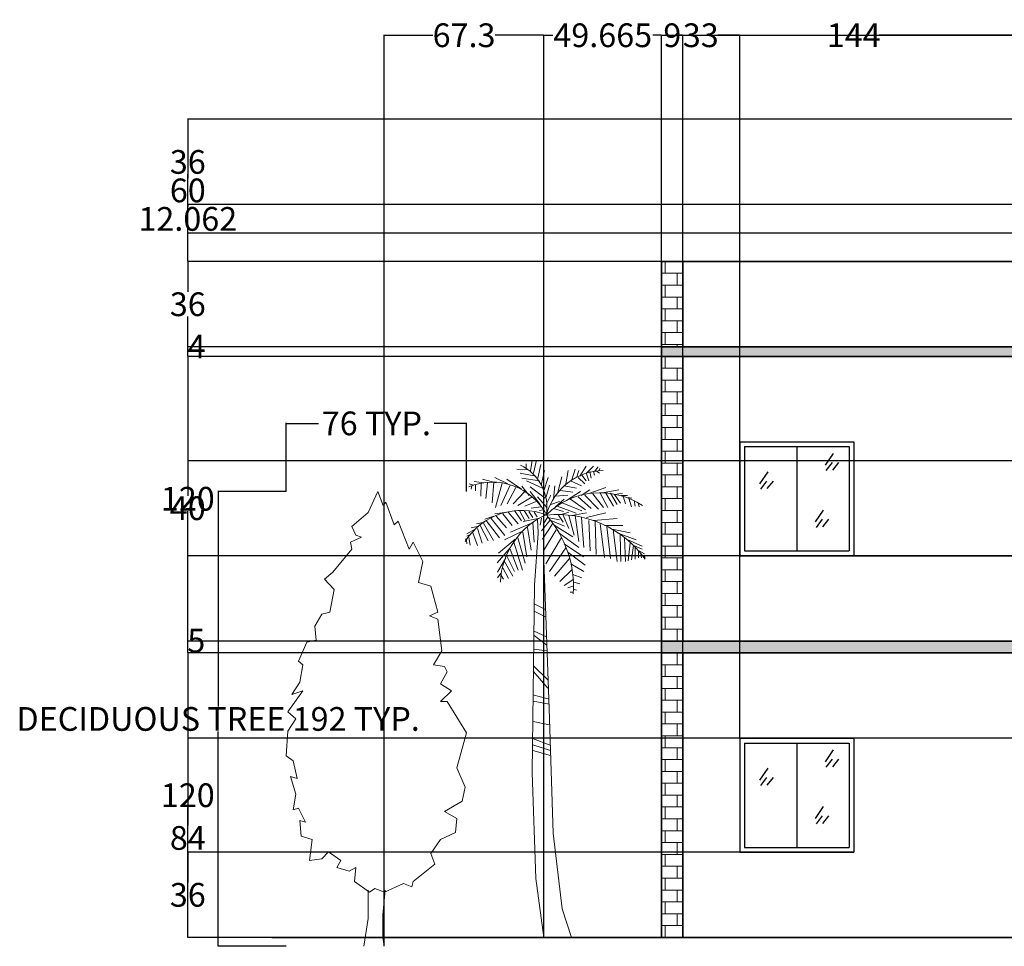
# Model space of a CAD drawing. Units: inches. Extents: x 403 to 1256, y 451 to 842.
# Tile 1 of 4: x 403 to 818, y 451 to 842. Entities that reach past the tile are written whole.
import ezdxf

# ---------------------------------------------------------------- set-up
doc = ezdxf.new("R2010")
doc.units = ezdxf.units.IN
doc.header["$MEASUREMENT"] = 0
for name, color, linetype, lineweight in [('A-ANNO-DIMS', 2, 'Continuous', 18), ('A-GLAZ', 4, 'Continuous', 25), ('A-WALL', 7, 'Continuous', 35), ('A-WALL-PATT', 8, 'Continuous', 13), ('PLANTS', 3, 'Continuous', 18)]:
    doc.layers.add(name, color=color, linetype=linetype, lineweight=lineweight)
doc.styles.get("Standard").update_dxf_attribs({"font": 'arial.ttf'})
doc.dimstyles.get("Standard").update_dxf_attribs({"dimtxt": 10, "dimasz": 0.18, "dimexe": 0.18, "dimexo": 0.0625, "dimgap": 0.09, "dimtad": 0, "dimtih": 1, "dimtoh": 1, "dimdec": 0, "dimzin": 0, "dimdsep": 46, "dimlunit": 3, "dimtxsty": 'Standard', "dimcen": 0.09, "dimadec": 0, "dimazin": 0, "dimtfac": 1, "dimtdec": 0, "dimtofl": 0, "dimtmove": 0, "dimatfit": 3, "dimfxl": 1, "dimtolj": 1, "dimtzin": 0, "dimarcsym": 0})
pattern_1 = [(50, (0, 0), (6.455342, -0.56477), [0.675, -7.425]), (355, (0, 0), (-1.248762, 6.76973), [0.54, -5.94]), (100.45144, (0.538, -0.047), (5.20658, 6.20496), [0.573662, -6.31028]), (46.1842, (0, 1.8), (9.60517, -1.489674), [1.0125, -11.1375]), (96.6356, (0.8, 1.676), (8.41196, 8.76707), [0.86049, -9.465424]), (351.1842, (0, 1.8), (8.41196, 8.76707), [0.81, -8.91]), (21, (0.9, 1.35), (5.372163, -3.62357), [0.675, -7.425]), (326, (0.9, 1.35), (2.189838, 6.52635), [0.54, -5.94]), (71.45144, (1.3477, 1.048), (7.562, 2.90278), [0.573662, -6.31028]), (37.5, (0, 0), (0.1094387, 2.9960447), [0, -5.868, 0, -6.03, 0, -5.9625]), (7.5, (0, 0), (2.367626, 3.549705), [0, -3.438, 0, -5.733, 0, -2.2725]), (327.5, (-2.007, 0), (4.804402, -0.202994), [0, -2.25, 0, -7.02, 0, -9.315]), (317.5, (-2.907, 0), (5.248676, 0.900945), [0, -2.925, 0, -4.662, 0, -6.615])]

# ---------------------------------------------------------------- blocks, each defined once
blk = doc.blocks.new('Tree - palm elevation')
for p, q in [((-7.5, 199.68), (-7.5, 197.946)), ((-5.567, 196.707), (-4.987, 201.167)), ((-4.407, 195.716), (-3.247, 200.672)), ((-2.474, 193.733), (-1.315, 199.433)), ((-6.727, 197.202), (-11.366, 197.45)), ((-3.441, 194.477), (-10.013, 195.716)), ((-1.121, 190.759), (0.232, 196.955)), ((9.317, 191.255), (10.283, 196.955)), ((11.829, 192.99), (13.182, 197.45)), ((13.956, 194.229), (14.729, 196.955)), ((15.116, 194.477), (17.822, 198.689)), ((18.015, 195.716), (20.914, 198.689)), ((18.015, 195.468), (18.981, 192.494)), ((19.368, 196.459), (19.948, 193.733)), ((20.914, 196.459), (21.301, 194.972)), ((21.301, 196.459), (22.847, 198.441)), ((22.074, 196.707), (23.427, 195.716)), ((23.234, 196.707), (23.62, 197.698)), ((-29.729, 190.759), (-31.469, 191.255)), ((-25.283, 191.751), (-29.342, 192.246)), ((-26.443, 191.503), (-26.636, 186.051)), ((-20.064, 191.751), (-25.863, 193.238)), ((-23.737, 191.751), (-24.51, 185.06)), ((-21.031, 191.998), (-21.804, 183.325)), ((-15.232, 191.255), (-20.644, 193.981)), ((-17.551, 191.503), (-20.451, 181.343)), ((-9.433, 189.025), (-15.618, 193.238)), ((-1.894, 192.494), (-9.24, 193.733)), ((-0.541, 189.52), (-7.307, 192.494)), ((0.038, 188.281), (1.778, 193.981)), ((5.837, 187.786), (7.577, 194.229)), ((11.25, 192.494), (15.889, 190.512)), ((14.536, 193.981), (17.242, 191.255)), ((16.082, 194.972), (17.822, 192.494)), ((-30.309, 190.512), (-30.695, 189.025)), ((-28.763, 190.759), (-28.763, 188.281)), ((-14.265, 190.759), (-18.131, 182.086)), ((-11.753, 189.768), (-15.425, 182.83)), ((-8.08, 188.034), (-12.912, 182.83)), ((-6.147, 186.299), (-9.24, 190.264)), ((-5.76, 190.016), (0.618, 185.308)), ((-5.76, 188.034), (-1.508, 182.582)), ((1.005, 185.803), (2.358, 190.759)), ((4.098, 185.06), (4.678, 190.512)), ((6.997, 188.529), (12.216, 187.786)), ((8.544, 190.512), (13.763, 189.52)), ((9.51, 184.317), (15.502, 188.034)), ((15.695, 186.299), (19.368, 188.777)), ((19.368, 187.29), (26.133, 189.768)), ((20.721, 187.042), (25.167, 181.343)), ((23.814, 187.29), (26.907, 181.343)), ((24.78, 187.538), (31.546, 188.777)), ((26.133, 187.29), (29.419, 181.838)), ((28.066, 187.29), (30.966, 182.582)), ((29.999, 186.795), (33.092, 187.29)), ((-4.987, 185.803), (-10.979, 182.086)), ((-3.247, 183.821), (-8.08, 181.838)), ((-2.668, 185.803), (1.198, 181.343)), ((1.005, 182.582), (2.938, 186.547)), ((2.938, 182.582), (6.61, 183.821)), ((4.871, 186.051), (10.09, 186.547)), ((4.871, 181.591), (8.544, 184.812)), ((7.77, 183.325), (16.082, 179.856)), ((11.25, 184.812), (17.628, 180.352)), ((14.536, 185.803), (19.948, 180.847)), ((17.242, 186.547), (23.041, 180.599)), ((29.806, 186.795), (32.319, 183.078)), ((32.512, 186.299), (35.218, 186.299)), ((33.479, 186.051), (34.445, 182.83)), ((35.605, 185.556), (37.151, 185.308)), ((35.798, 185.308), (36.958, 181.591)), ((38.118, 184.317), (38.504, 181.838)), ((39.857, 182.83), (40.244, 181.591)), ((-15.618, 179.36), (-20.644, 178.617)), ((-17.358, 178.617), (-13.299, 173.661)), ((-15.038, 179.36), (-10.786, 174.404)), ((-12.332, 180.104), (-9.433, 175.643)), ((-10.206, 180.104), (-8.08, 175.891)), ((-8.273, 180.104), (-6.147, 176.635)), ((-6.34, 179.608), (-4.6, 177.13)), ((-1.315, 181.591), (-5.374, 181.095)), ((-4.021, 179.36), (-2.861, 177.378)), ((-0.348, 180.352), (-1.894, 180.104)), ((4.098, 180.847), (8.35, 179.608)), ((5.644, 181.838), (13.569, 178.865)), ((7.384, 178.369), (10.476, 179.36)), ((11.829, 177.874), (18.015, 179.113)), ((18.015, 177.13), (26.133, 179.113)), ((-25.09, 175.148), (-28.376, 174.404)), ((-25.476, 174.652), (-21.224, 167.466)), ((-21.031, 177.626), (-24.897, 176.387)), ((-24.317, 175.891), (-18.711, 168.457)), ((-22.191, 176.635), (-16.391, 169.448)), ((-20.064, 177.626), (-15.812, 172.67)), ((-4.214, 175.148), (-14.072, 170.935)), ((-1.701, 176.882), (-8.66, 175.396)), ((-4.6, 174.9), (-4.021, 166.722)), ((-2.668, 176.387), (-2.376, 170.594)), ((-0.928, 176.882), (-1.508, 173.909)), ((2.551, 175.891), (-0.928, 171.431)), ((3.711, 174.404), (-0.541, 167.961)), ((1.585, 177.13), (0.038, 174.652)), ((1.585, 177.13), (6.61, 176.139)), ((2.938, 175.891), (8.737, 173.413)), ((6.224, 178.121), (8.157, 175.148)), ((8.157, 178.121), (10.476, 172.422)), ((10.476, 177.874), (12.796, 169.696)), ((13.182, 177.874), (14.729, 166.97)), ((15.889, 177.13), (16.855, 164.492)), ((18.981, 175.891), (19.561, 163.005)), ((20.914, 175.891), (30.966, 176.635)), ((21.688, 175.396), (22.074, 161.518)), ((23.814, 174.404), (25.554, 160.279)), ((-28.956, 172.174), (-32.435, 170.192)), ((-27.409, 173.413), (-30.695, 172.67)), ((-29.922, 170.687), (-27.989, 165.235)), ((-27.989, 172.422), (-26.056, 166.227)), ((-26.829, 173.661), (-23.544, 167.218)), ((-8.466, 171.678), (-16.585, 167.713)), ((-8.853, 170.935), (-7.113, 160.527)), ((-6.92, 172.917), (-5.374, 163.253)), ((5.257, 171.926), (-0.155, 163.005)), ((4.291, 173.909), (12.216, 168.953)), ((6.417, 170.439), (14.729, 164.492)), ((25.554, 173.661), (33.285, 173.661)), ((26.52, 173.165), (28.066, 159.784)), ((28.839, 172.174), (36.378, 170.687)), ((29.226, 171.926), (30.966, 158.545)), ((30.966, 170.687), (38.891, 167.713)), ((-32.628, 167.961), (-33.208, 167.961)), ((-32.628, 167.713), (-32.435, 165.979)), ((-31.082, 169.944), (-32.435, 169.2)), ((-31.662, 168.705), (-31.082, 165.483)), ((-12.139, 167.961), (-19.098, 162.014)), ((-12.719, 166.722), (-9.046, 154.828)), ((-10.979, 168.457), (-7.887, 157.801)), ((7.384, 168.705), (0.812, 157.553)), ((32.126, 169.696), (32.512, 158.545)), ((34.058, 168.705), (34.445, 158.545)), ((35.412, 167.713), (41.404, 164.988)), ((36.378, 166.474), (35.605, 158.792)), ((-14.265, 164.244), (-19.678, 158.049)), ((-14.265, 163.749), (-10.786, 154.828)), ((9.317, 164.244), (2.358, 154.332)), ((8.544, 165.979), (16.662, 160.527)), ((10.09, 162.51), (17.435, 157.058)), ((37.731, 165.235), (36.958, 159.288)), ((37.924, 165.235), (41.404, 163.749)), ((38.504, 164.492), (38.504, 159.536)), ((39.664, 163.253), (42.37, 161.766)), ((39.857, 162.757), (39.857, 160.031)), ((-16.005, 160.031), (-19.484, 154.084)), ((-16.585, 158.545), (-13.106, 152.35)), ((-15.618, 160.775), (-12.332, 154.332)), ((10.863, 159.784), (4.484, 152.35)), ((40.824, 161.766), (41.21, 160.031)), ((41.21, 161.518), (42.757, 160.279)), ((-17.358, 155.819), (-14.845, 151.358)), ((11.829, 155.075), (6.804, 150.119)), ((11.443, 157.553), (16.855, 154.332)), ((-18.131, 153.589), (-19.484, 151.606)), ((-17.938, 152.597), (-16.972, 151.111)), ((12.603, 151.111), (8.544, 148.385)), ((12.216, 153.093), (16.082, 151.606)), ((12.603, 149.872), (15.116, 149.128)), ((12.216, 148.137), (10.09, 147.393)), ((12.409, 145.659), (11.056, 145.659)), ((12.409, 146.898), (13.763, 146.402)), ((-4.081, 140.645), (0.753, 138.261)), ((-4.081, 137.547), (0.753, 135.163)), ((-4.081, 129.205), (1.124, 126.821)), ((-4.081, 127.298), (1.31, 123.246)), ((-4.081, 121.578), (1.31, 120.863)), ((-4.453, 112.283), (1.682, 105.133)), ((-4.267, 114.428), (1.682, 108.708)), ((-4.639, 102.273), (1.868, 100.604)), ((-4.453, 99.651), (2.24, 98.459)), ((-4.453, 91.071), (2.426, 89.641)), ((-4.825, 83.921), (2.612, 81.061)), ((-4.639, 81.299), (2.797, 78.916)), ((-4.639, 78.916), (2.797, 76.771))]:
    blk.add_line(p, q)
for points in [[(-2.363, 170.553), (-3.88, 148.505), (-4.988, 69.634), (-3.325, 24.869), (0, 0)], [(-0.116, 162.848), (0.554, 143.532), (2.217, 96.635), (3.88, 44.054), (7.76, 12.079), (11.64, 0)]]:
    blk.add_lwpolyline(points)
for centre, radius, start, end in [((-18.427, 181.448), 19.715, 350.285, 64.11229), ((25.595, 171.567), 25.395, 91.40319, 163.882), ((-21.738, 166.094), 25.899, 27.67115, 112.5305), ((23.687, 155.341), 32.188, 56.19272, 134.3213), ((-9.259, 151.732), 28.386, 68.38311, 147.5322), ((14.394, 148.393), 32.752, 113.7592, 177.4133), ((5.828, 132.718), 45.639, 35.98777, 95.82273), ((-32.8, 147.923), 45.309, 356.1943, 41.37848)]:
    blk.add_arc(centre, radius, start, end)
blk = doc.blocks.new('Tree - type 2 deciduous elevation')
blk.add_lwpolyline([(-2.754, 191.699), (-6.78, 182.851), (-13.682, 176.953), (-11.956, 173.266), (-9.656, 172.529), (-14.257, 170.317), (-13.682, 167.368), (-21.733, 157.783), (-25.184, 154.834), (-21.158, 150.41), (-21.733, 147.461), (-22.884, 140.825), (-26.334, 140.087), (-29.21, 134.926), (-28.635, 129.028), (-32.661, 128.291), (-36.111, 120.18), (-34.386, 118.706), (-35.536, 111.333), (-38.987, 106.171), (-34.386, 107.646), (-40.712, 98.798), (-37.261, 95.849), (-40.712, 90.688), (-41.287, 80.366), (-38.412, 78.154), (-36.686, 70.781), (-39.562, 71.518), (-37.261, 64.145), (-38.412, 57.509), (-36.111, 58.247), (-33.236, 52.348), (-35.536, 53.086), (-34.961, 46.45), (-30.36, 44.975), (-31.51, 36.128), (-26.334, 36.865), (-23.459, 39.814), (-18.283, 36.128), (-20.008, 33.178), (-14.832, 31.704), (-11.956, 33.178), (-12.531, 27.28), (-6.205, 22.856), (-3.905, 24.331), (0.121, 22.856), (8.173, 26.543), (11.624, 25.068), (12.199, 27.28), (21.4, 34.653), (19.675, 39.077), (23.701, 44.975), (30.027, 47.924), (30.602, 53.823), (25.426, 56.772), (32.903, 61.196), (34.053, 67.094), (30.602, 75.205), (34.628, 89.951), (26.576, 103.222), (23.701, 103.222), (28.302, 107.646), (23.701, 110.595), (26.576, 115.756), (25.426, 117.968), (20.825, 118.706), (24.276, 124.604), (22.551, 137.876), (19.1, 139.35), (22.551, 140.825), (19.675, 151.884), (14.499, 153.359), (16.224, 162.207), (12.199, 170.317), (10.473, 167.368), (5.872, 179.165), (4.147, 177.69), (0.696, 187.275), (-0.454, 185.8)], close=True)
for points in [[(-6.813, 23.669), (-6.813, 11.669), (-8.627, 0)], [(0.387, 23.669), (-0.576, 13.271), (-0.576, 3.686), (0, 0)]]:
    blk.add_lwpolyline(points)
blk = doc.blocks.new('WIN-1200')
for p, q in [((0, 48), (0, 0)), ((0, 48), (48, 48)), ((2, 46), (46, 46)), ((2, 46), (2, 2)), ((24, 46), (24, 2)), ((46, 46), (46, 2)), ((48, 48), (48, 0)), ((39.35, 43.11), (35.96, 38.1)), ((38.86, 39.23), (36.28, 35.84)), ((41.61, 39.23), (39.03, 36)), ((11.71, 35.36), (8.32, 30.35)), ((11.23, 31.48), (8.64, 28.09)), ((13.98, 31.48), (11.39, 28.25)), ((35.15, 19.21), (31.75, 14.2)), ((34.66, 15.33), (32.08, 11.94)), ((37.41, 15.33), (34.82, 12.1)), ((2, 2), (46, 2)), ((0, 0), (48, 0))]:
    blk.add_line(p, q)
blk = doc.blocks.new('*D9')
at = {"layer": 'A-ANNO-DIMS', "color": 0, "lineweight": -2, "transparency": 16777216}
for p, q in [((515.15, 642.97), (486.28, 642.97)), ((486.46, 642.79), (486.46, 552.39)), ((486.46, 451.46), (486.46, 541.86)), ((515.15, 451.28), (486.28, 451.28))]:
    blk.add_line(p, q, dxfattribs=at)
at = {"layer": 'A-ANNO-DIMS', "color": 0, "transparency": 16777216}
for points in [[(486.43, 642.79), (486.49, 642.79), (486.46, 642.97)], [(486.43, 451.46), (486.49, 451.46), (486.46, 451.28)]]:
    blk.add_solid(points, dxfattribs=at)
at = {"layer": 'Defpoints', "color": 0, "transparency": 16777216}
for p in [(486.46, 642.97), (515.21, 642.97), (515.21, 451.28)]:
    blk.add_point(p, dxfattribs=at)
at = {"layer": 'A-ANNO-DIMS', "color": 0, "transparency": 16777216, "insert": (486.46, 547.13), "char_height": 10, "attachment_point": 5}
blk.add_mtext('\\A1;DECIDUOUS TREE 192 TYP.', dxfattribs=at)
blk = doc.blocks.new('*D10')
at = {"layer": 'A-ANNO-DIMS', "color": 0, "lineweight": -2, "transparency": 16777216}
for p, q in [((515.21, 643.04), (515.21, 671.91)), ((515.39, 671.73), (528.78, 671.73)), ((590.95, 671.73), (577.56, 671.73)), ((591.13, 643.04), (591.13, 671.91))]:
    blk.add_line(p, q, dxfattribs=at)
at = {"layer": 'A-ANNO-DIMS', "color": 0, "transparency": 16777216}
for points in [[(515.39, 671.76), (515.39, 671.7), (515.21, 671.73)], [(590.95, 671.76), (590.95, 671.7), (591.13, 671.73)]]:
    blk.add_solid(points, dxfattribs=at)
at = {"layer": 'Defpoints', "color": 0, "transparency": 16777216}
for p in [(591.13, 671.73), (515.21, 642.97), (591.13, 642.97)]:
    blk.add_point(p, dxfattribs=at)
at = {"layer": 'A-ANNO-DIMS', "color": 0, "transparency": 16777216, "insert": (553.17, 671.73), "char_height": 10, "attachment_point": 5}
blk.add_mtext('\\A1;76 TYP.', dxfattribs=at)
blk = doc.blocks.new('*D11')
at = {"layer": 'A-ANNO-DIMS', "color": 0, "lineweight": -2, "transparency": 16777216}
for p, q in [((673.46, 704.02), (673.46, 835.54)), ((673.64, 835.36), (846.82, 835.36)), ((1042.28, 835.36), (869.1, 835.36)), ((1042.46, 704.02), (1042.46, 835.54))]:
    blk.add_line(p, q, dxfattribs=at)
at = {"layer": 'A-ANNO-DIMS', "color": 0, "transparency": 16777216}
for points in [[(673.64, 835.39), (673.64, 835.33), (673.46, 835.36)], [(1042.28, 835.39), (1042.28, 835.33), (1042.46, 835.36)]]:
    blk.add_solid(points, dxfattribs=at)
at = {"layer": 'Defpoints', "color": 0, "transparency": 16777216}
for p in [(1042.46, 835.36), (673.46, 703.96), (1042.46, 703.96)]:
    blk.add_point(p, dxfattribs=at)
at = {"layer": 'A-ANNO-DIMS', "color": 0, "transparency": 16777216, "insert": (857.96, 835.36), "char_height": 10, "attachment_point": 5}
blk.add_mtext('\\A1;369', dxfattribs=at)
blk = doc.blocks.new('*D13')
at = {"layer": 'A-ANNO-DIMS', "color": 0, "lineweight": -2, "transparency": 16777216}
for p, q in [((673.4, 574.96), (473.5, 574.96)), ((473.68, 574.78), (473.68, 520.16)), ((473.68, 455.14), (473.68, 509.77)), ((673.4, 454.96), (473.5, 454.96))]:
    blk.add_line(p, q, dxfattribs=at)
at = {"layer": 'A-ANNO-DIMS', "color": 0, "transparency": 16777216}
for points in [[(473.65, 574.78), (473.71, 574.78), (473.68, 574.96)], [(473.65, 455.14), (473.71, 455.14), (473.68, 454.96)]]:
    blk.add_solid(points, dxfattribs=at)
at = {"layer": 'Defpoints', "color": 0, "transparency": 16777216}
for p in [(473.68, 574.96), (673.46, 574.96), (673.46, 454.96)]:
    blk.add_point(p, dxfattribs=at)
at = {"layer": 'A-ANNO-DIMS', "color": 0, "transparency": 16777216, "insert": (473.68, 514.96), "char_height": 10, "attachment_point": 5}
blk.add_mtext('\\A1;120', dxfattribs=at)
blk = doc.blocks.new('*D14')
at = {"layer": 'A-ANNO-DIMS', "color": 0, "lineweight": -2, "transparency": 16777216}
for p, q in [((673.4, 579.96), (473.5, 579.96)), ((473.68, 579.96), (473.68, 580.14)), ((473.68, 580.14), (473.86, 580.14)), ((473.68, 575.14), (473.68, 579.78)), ((673.4, 574.96), (473.5, 574.96))]:
    blk.add_line(p, q, dxfattribs=at)
at = {"layer": 'A-ANNO-DIMS', "color": 0, "transparency": 16777216}
for points in [[(473.65, 579.78), (473.71, 579.78), (473.68, 579.96)], [(473.65, 575.14), (473.71, 575.14), (473.68, 574.96)]]:
    blk.add_solid(points, dxfattribs=at)
at = {"layer": 'Defpoints', "color": 0, "transparency": 16777216}
for p in [(473.68, 579.96), (673.46, 579.96), (673.46, 574.96)]:
    blk.add_point(p, dxfattribs=at)
at = {"layer": 'A-ANNO-DIMS', "color": 0, "transparency": 16777216, "insert": (477.27, 580.14), "char_height": 10, "attachment_point": 5}
blk.add_mtext('\\A1;5', dxfattribs=at)
blk = doc.blocks.new('*D15')
at = {"layer": 'A-ANNO-DIMS', "color": 0, "lineweight": -2, "transparency": 16777216}
for p, q in [((673.4, 699.96), (473.5, 699.96)), ((473.68, 699.78), (473.68, 645.16)), ((473.68, 580.14), (473.68, 634.77)), ((673.4, 579.96), (473.5, 579.96))]:
    blk.add_line(p, q, dxfattribs=at)
at = {"layer": 'A-ANNO-DIMS', "color": 0, "transparency": 16777216}
for points in [[(473.65, 699.78), (473.71, 699.78), (473.68, 699.96)], [(473.65, 580.14), (473.71, 580.14), (473.68, 579.96)]]:
    blk.add_solid(points, dxfattribs=at)
at = {"layer": 'Defpoints', "color": 0, "transparency": 16777216}
for p in [(473.68, 699.96), (673.46, 699.96), (673.46, 579.96)]:
    blk.add_point(p, dxfattribs=at)
at = {"layer": 'A-ANNO-DIMS', "color": 0, "transparency": 16777216, "insert": (473.68, 639.96), "char_height": 10, "attachment_point": 5}
blk.add_mtext('\\A1;120', dxfattribs=at)
blk = doc.blocks.new('*D16')
at = {"layer": 'A-ANNO-DIMS', "color": 0, "lineweight": -2, "transparency": 16777216}
for p, q in [((673.4, 703.96), (473.5, 703.96)), ((473.68, 703.96), (473.68, 704.14)), ((473.68, 704.14), (473.86, 704.14)), ((473.68, 700.14), (473.68, 703.78)), ((673.4, 699.96), (473.5, 699.96))]:
    blk.add_line(p, q, dxfattribs=at)
at = {"layer": 'A-ANNO-DIMS', "color": 0, "transparency": 16777216}
for points in [[(473.65, 703.78), (473.71, 703.78), (473.68, 703.96)], [(473.65, 700.14), (473.71, 700.14), (473.68, 699.96)]]:
    blk.add_solid(points, dxfattribs=at)
at = {"layer": 'Defpoints', "color": 0, "transparency": 16777216}
for p in [(473.68, 703.96), (673.46, 703.96), (673.46, 699.96)]:
    blk.add_point(p, dxfattribs=at)
at = {"layer": 'A-ANNO-DIMS', "color": 0, "transparency": 16777216, "insert": (477.41, 704.14), "char_height": 10, "attachment_point": 5}
blk.add_mtext('\\A1;4', dxfattribs=at)
blk = doc.blocks.new('*D17')
at = {"layer": 'A-ANNO-DIMS', "color": 0, "lineweight": -2, "transparency": 16777216}
for p, q in [((673.4, 739.96), (473.5, 739.96)), ((473.68, 739.78), (473.68, 727.16)), ((473.68, 704.14), (473.68, 716.76)), ((673.4, 703.96), (473.5, 703.96))]:
    blk.add_line(p, q, dxfattribs=at)
at = {"layer": 'A-ANNO-DIMS', "color": 0, "transparency": 16777216}
for points in [[(473.65, 739.78), (473.71, 739.78), (473.68, 739.96)], [(473.65, 704.14), (473.71, 704.14), (473.68, 703.96)]]:
    blk.add_solid(points, dxfattribs=at)
at = {"layer": 'Defpoints', "color": 0, "transparency": 16777216}
for p in [(473.68, 739.96), (673.46, 739.96), (673.46, 703.96)]:
    blk.add_point(p, dxfattribs=at)
at = {"layer": 'A-ANNO-DIMS', "color": 0, "transparency": 16777216, "insert": (473.68, 721.96), "char_height": 10, "attachment_point": 5}
blk.add_mtext('\\A1;36', dxfattribs=at)
blk = doc.blocks.new('*D18')
at = {"layer": 'A-ANNO-DIMS', "color": 0, "lineweight": -2, "transparency": 16777216}
for p, q in [((965.9, 799.96), (473.5, 799.96)), ((473.68, 799.78), (473.68, 775.16)), ((473.68, 740.14), (473.68, 764.77)), ((673.4, 739.96), (473.5, 739.96))]:
    blk.add_line(p, q, dxfattribs=at)
at = {"layer": 'A-ANNO-DIMS', "color": 0, "transparency": 16777216}
for points in [[(473.65, 799.78), (473.71, 799.78), (473.68, 799.96)], [(473.65, 740.14), (473.71, 740.14), (473.68, 739.96)]]:
    blk.add_solid(points, dxfattribs=at)
at = {"layer": 'Defpoints', "color": 0, "transparency": 16777216}
for p in [(473.68, 799.96), (965.96, 799.96), (673.46, 739.96)]:
    blk.add_point(p, dxfattribs=at)
at = {"layer": 'A-ANNO-DIMS', "color": 0, "transparency": 16777216, "insert": (473.68, 769.96), "char_height": 10, "attachment_point": 5}
blk.add_mtext('\\A1;60', dxfattribs=at)
blk = doc.blocks.new('*D19')
at = {"layer": 'A-ANNO-DIMS', "color": 0, "lineweight": -2, "transparency": 16777216}
for p, q in [((754.4, 490.96), (473.5, 490.96)), ((473.68, 490.78), (473.68, 478.16)), ((473.68, 455.14), (473.68, 467.76)), ((826.4, 454.96), (473.5, 454.96))]:
    blk.add_line(p, q, dxfattribs=at)
at = {"layer": 'A-ANNO-DIMS', "color": 0, "transparency": 16777216}
for points in [[(473.65, 490.78), (473.71, 490.78), (473.68, 490.96)], [(473.65, 455.14), (473.71, 455.14), (473.68, 454.96)]]:
    blk.add_solid(points, dxfattribs=at)
at = {"layer": 'Defpoints', "color": 0, "transparency": 16777216}
for p in [(754.46, 490.96), (473.68, 454.96), (826.46, 454.96)]:
    blk.add_point(p, dxfattribs=at)
at = {"layer": 'A-ANNO-DIMS', "color": 0, "transparency": 16777216, "insert": (473.68, 472.96), "char_height": 10, "attachment_point": 5}
blk.add_mtext('\\A1;36', dxfattribs=at)
blk = doc.blocks.new('*D20')
at = {"layer": 'A-ANNO-DIMS', "color": 0, "lineweight": -2, "transparency": 16777216}
for p, q in [((706.52, 615.96), (1244.44, 615.96)), ((1244.26, 615.78), (1244.26, 603.16)), ((1244.26, 580.14), (1244.26, 592.76)), ((682.52, 579.96), (1244.44, 579.96))]:
    blk.add_line(p, q, dxfattribs=at)
at = {"layer": 'A-ANNO-DIMS', "color": 0, "transparency": 16777216}
for points in [[(1244.23, 615.78), (1244.29, 615.78), (1244.26, 615.96)], [(1244.23, 580.14), (1244.29, 580.14), (1244.26, 579.96)]]:
    blk.add_solid(points, dxfattribs=at)
at = {"layer": 'Defpoints', "color": 0, "transparency": 16777216}
for p in [(706.46, 615.96), (1244.26, 615.96), (682.46, 579.96)]:
    blk.add_point(p, dxfattribs=at)
at = {"layer": 'A-ANNO-DIMS', "color": 0, "transparency": 16777216, "insert": (1244.26, 597.96), "char_height": 10, "attachment_point": 5}
blk.add_mtext('\\A1;36', dxfattribs=at)
blk = doc.blocks.new('*D21')
at = {"layer": 'A-ANNO-DIMS', "color": 0, "lineweight": -2, "transparency": 16777216}
for p, q in [((673.46, 455.02), (673.46, 835.54)), ((673.64, 835.36), (682.71, 835.36)), ((706.28, 835.36), (697.21, 835.36)), ((706.46, 539.02), (706.46, 835.54))]:
    blk.add_line(p, q, dxfattribs=at)
at = {"layer": 'A-ANNO-DIMS', "color": 0, "transparency": 16777216}
for points in [[(673.64, 835.39), (673.64, 835.33), (673.46, 835.36)], [(706.28, 835.39), (706.28, 835.33), (706.46, 835.36)]]:
    blk.add_solid(points, dxfattribs=at)
at = {"layer": 'Defpoints', "color": 0, "transparency": 16777216}
for p in [(706.46, 835.36), (706.46, 538.96), (673.46, 454.96)]:
    blk.add_point(p, dxfattribs=at)
at = {"layer": 'A-ANNO-DIMS', "color": 0, "transparency": 16777216, "insert": (689.96, 835.36), "char_height": 10, "attachment_point": 5}
blk.add_mtext('\\A1;33', dxfattribs=at)
blk = doc.blocks.new('*D23')
at = {"layer": 'A-ANNO-DIMS', "color": 0, "lineweight": -2, "transparency": 16777216}
for p, q in [((682.46, 455.02), (682.46, 835.54)), ((682.64, 835.36), (743.81, 835.36)), ((826.28, 835.36), (765.1, 835.36)), ((826.46, 455.02), (826.46, 835.54))]:
    blk.add_line(p, q, dxfattribs=at)
at = {"layer": 'A-ANNO-DIMS', "color": 0, "transparency": 16777216}
for points in [[(682.64, 835.39), (682.64, 835.33), (682.46, 835.36)], [(826.28, 835.39), (826.28, 835.33), (826.46, 835.36)]]:
    blk.add_solid(points, dxfattribs=at)
at = {"layer": 'Defpoints', "color": 0, "transparency": 16777216}
for p in [(826.46, 835.36), (682.46, 454.96), (826.46, 454.96)]:
    blk.add_point(p, dxfattribs=at)
at = {"layer": 'A-ANNO-DIMS', "color": 0, "transparency": 16777216, "insert": (754.46, 835.36), "char_height": 10, "attachment_point": 5}
blk.add_mtext('\\A1;144', dxfattribs=at)
blk = doc.blocks.new('*D28')
at = {"layer": 'A-ANNO-DIMS', "color": 0, "lineweight": -2, "transparency": 16777216}
for p, q in [((556.5, 451.34), (556.5, 835.54)), ((556.68, 835.36), (577.04, 835.36)), ((623.61, 835.36), (603.25, 835.36)), ((623.79, 455.02), (623.79, 835.54))]:
    blk.add_line(p, q, dxfattribs=at)
at = {"layer": 'A-ANNO-DIMS', "color": 0, "transparency": 16777216}
for points in [[(556.68, 835.39), (556.68, 835.33), (556.5, 835.36)], [(623.61, 835.39), (623.61, 835.33), (623.79, 835.36)]]:
    blk.add_solid(points, dxfattribs=at)
at = {"layer": 'Defpoints', "color": 0, "transparency": 16777216}
for p in [(623.79, 835.36), (623.79, 454.96), (556.5, 451.28)]:
    blk.add_point(p, dxfattribs=at)
at = {"layer": 'A-ANNO-DIMS', "color": 0, "transparency": 16777216, "insert": (590.15, 835.36), "char_height": 10, "attachment_point": 5}
blk.add_mtext('\\A1;67.3', dxfattribs=at)
blk = doc.blocks.new('*D29')
at = {"layer": 'A-ANNO-DIMS', "color": 0, "lineweight": -2, "transparency": 16777216}
for p, q in [((623.79, 455.02), (623.79, 835.54)), ((623.97, 835.36), (627.54, 835.36)), ((673.28, 835.36), (669.71, 835.36)), ((673.46, 455.02), (673.46, 835.54))]:
    blk.add_line(p, q, dxfattribs=at)
at = {"layer": 'A-ANNO-DIMS', "color": 0, "transparency": 16777216}
for points in [[(623.97, 835.39), (623.97, 835.33), (623.79, 835.36)], [(673.28, 835.39), (673.28, 835.33), (673.46, 835.36)]]:
    blk.add_solid(points, dxfattribs=at)
at = {"layer": 'Defpoints', "color": 0, "transparency": 16777216}
for p in [(673.46, 835.36), (623.79, 454.96), (673.46, 454.96)]:
    blk.add_point(p, dxfattribs=at)
at = {"layer": 'A-ANNO-DIMS', "color": 0, "transparency": 16777216, "insert": (648.63, 835.36), "char_height": 10, "attachment_point": 5}
blk.add_mtext('\\A1;49.665', dxfattribs=at)
blk = doc.blocks.new('*D33')
at = {"layer": 'A-ANNO-DIMS', "color": 0, "lineweight": -2, "transparency": 16777216}
for p, q in [((830.4, 538.96), (473.5, 538.96)), ((473.68, 538.78), (473.68, 502.16)), ((473.68, 455.14), (473.68, 491.77)), ((830.4, 454.96), (473.5, 454.96))]:
    blk.add_line(p, q, dxfattribs=at)
at = {"layer": 'A-ANNO-DIMS', "color": 0, "transparency": 16777216}
for points in [[(473.65, 538.78), (473.71, 538.78), (473.68, 538.96)], [(473.65, 455.14), (473.71, 455.14), (473.68, 454.96)]]:
    blk.add_solid(points, dxfattribs=at)
at = {"layer": 'Defpoints', "color": 0, "transparency": 16777216}
for p in [(473.68, 538.96), (830.46, 538.96), (830.46, 454.96)]:
    blk.add_point(p, dxfattribs=at)
at = {"layer": 'A-ANNO-DIMS', "color": 0, "transparency": 16777216, "insert": (473.68, 496.96), "char_height": 10, "attachment_point": 5}
blk.add_mtext('\\A1;84', dxfattribs=at)
blk = doc.blocks.new('*D39')
at = {"layer": 'A-ANNO-DIMS', "color": 0, "lineweight": -2, "transparency": 16777216}
for p, q in [((860.4, 655.96), (473.5, 655.96)), ((473.68, 655.78), (473.68, 641.16)), ((473.68, 616.14), (473.68, 630.77)), ((860.4, 615.96), (473.5, 615.96))]:
    blk.add_line(p, q, dxfattribs=at)
at = {"layer": 'A-ANNO-DIMS', "color": 0, "transparency": 16777216}
for points in [[(473.65, 655.78), (473.71, 655.78), (473.68, 655.96)], [(473.65, 616.14), (473.71, 616.14), (473.68, 615.96)]]:
    blk.add_solid(points, dxfattribs=at)
at = {"layer": 'Defpoints', "color": 0, "transparency": 16777216}
for p in [(473.68, 655.96), (860.46, 655.96), (860.46, 615.96)]:
    blk.add_point(p, dxfattribs=at)
at = {"layer": 'A-ANNO-DIMS', "color": 0, "transparency": 16777216, "insert": (473.68, 635.96), "char_height": 10, "attachment_point": 5}
blk.add_mtext('\\A1;40', dxfattribs=at)
blk = doc.blocks.new('*D42')
at = {"layer": 'A-ANNO-DIMS', "color": 0, "lineweight": -2, "transparency": 16777216}
for p, q in [((673.46, 740.02), (673.46, 835.54)), ((673.64, 835.36), (674.58, 835.36)), ((682.28, 835.36), (681.34, 835.36)), ((682.46, 740.02), (682.46, 835.54))]:
    blk.add_line(p, q, dxfattribs=at)
at = {"layer": 'A-ANNO-DIMS', "color": 0, "transparency": 16777216}
for points in [[(673.64, 835.39), (673.64, 835.33), (673.46, 835.36)], [(682.28, 835.39), (682.28, 835.33), (682.46, 835.36)]]:
    blk.add_solid(points, dxfattribs=at)
at = {"layer": 'Defpoints', "color": 0, "transparency": 16777216}
for p in [(682.46, 835.36), (673.46, 739.96), (682.46, 739.96)]:
    blk.add_point(p, dxfattribs=at)
at = {"layer": 'A-ANNO-DIMS', "color": 0, "transparency": 16777216, "insert": (677.96, 835.36), "char_height": 10, "attachment_point": 5}
blk.add_mtext('\\A1;9', dxfattribs=at)
blk = doc.blocks.new('*D48')
at = {"layer": 'A-ANNO-DIMS', "color": 0, "lineweight": -2, "transparency": 16777216}
for p, q in [((889.4, 763.96), (473.5, 763.96)), ((473.68, 763.78), (473.68, 763.13)), ((868.49, 751.9), (473.5, 751.9)), ((473.68, 752.08), (473.68, 752.73))]:
    blk.add_line(p, q, dxfattribs=at)
at = {"layer": 'A-ANNO-DIMS', "color": 0, "transparency": 16777216}
for points in [[(473.65, 763.78), (473.71, 763.78), (473.68, 763.96)], [(473.65, 752.08), (473.71, 752.08), (473.68, 751.9)]]:
    blk.add_solid(points, dxfattribs=at)
at = {"layer": 'Defpoints', "color": 0, "transparency": 16777216}
for p in [(473.68, 763.96), (889.46, 763.96), (868.55, 751.9)]:
    blk.add_point(p, dxfattribs=at)
at = {"layer": 'A-ANNO-DIMS', "color": 0, "transparency": 16777216, "insert": (473.68, 757.93), "char_height": 10, "attachment_point": 5}
blk.add_mtext('\\A1;12.062', dxfattribs=at)
blk = doc.blocks.new('*D49')
at = {"layer": 'A-ANNO-DIMS', "color": 0, "lineweight": -2, "transparency": 16777216}
for p, q in [((965.9, 799.96), (473.5, 799.96)), ((473.68, 799.78), (473.68, 787.16)), ((473.68, 764.14), (473.68, 776.76)), ((889.4, 763.96), (473.5, 763.96))]:
    blk.add_line(p, q, dxfattribs=at)
at = {"layer": 'A-ANNO-DIMS', "color": 0, "transparency": 16777216}
for points in [[(473.65, 799.78), (473.71, 799.78), (473.68, 799.96)], [(473.65, 764.14), (473.71, 764.14), (473.68, 763.96)]]:
    blk.add_solid(points, dxfattribs=at)
at = {"layer": 'Defpoints', "color": 0, "transparency": 16777216}
for p in [(473.68, 799.96), (965.96, 799.96), (889.46, 763.96)]:
    blk.add_point(p, dxfattribs=at)
at = {"layer": 'A-ANNO-DIMS', "color": 0, "transparency": 16777216, "insert": (473.68, 781.96), "char_height": 10, "attachment_point": 5}
blk.add_mtext('\\A1;36', dxfattribs=at)

msp = doc.modelspace()

# ---------------------------------------------------------------- hatches: boundary and pattern name
at = {"layer": 'A-WALL-PATT'}
h = msp.add_hatch(dxfattribs=at)
h.set_pattern_fill('BRICK', color=256, scale=20)
h.paths.add_polyline_path([(673.459, 703.9615), (682.459, 703.9615), (682.459, 739.9615), (673.459, 739.9615)])
h.paths.add_polyline_path([(682.459, 699.9615), (673.459, 699.9615), (673.459, 579.9615), (682.459, 579.9615)])
h.paths.add_polyline_path([(673.459, 454.9615), (682.459, 454.9615), (682.459, 574.9615), (673.459, 574.9615)])
h.paths.add_polyline_path([(1031.459, 579.9615), (1042.459, 579.9615), (1042.459, 615.9615), (1042.459, 699.9615), (1033.459, 699.9615), (1031.459, 699.9615)])
h = msp.add_hatch(dxfattribs=at)
h.set_pattern_fill('AR-CONC', color=256, scale=0.9)
h.set_pattern_definition(pattern_1)
h.paths.add_polyline_path([(673.459, 703.9615), (673.459, 699.9615), (1033.459, 699.9615), (1042.459, 699.9615), (1042.459, 703.9615), (1033.459, 703.9615)])
h = msp.add_hatch(dxfattribs=at)
h.set_pattern_fill('AR-CONC', color=256, scale=0.9)
h.set_pattern_definition(pattern_1)
h.paths.add_polyline_path([(1042.459, 574.9615), (1042.459, 579.9615), (673.459, 579.9615), (673.459, 574.9615)])

# ---------------------------------------------------------------- linework, layer by layer
at = {"layer": 'A-WALL'}
for p, q in [((673.459, 739.9615), (673.459, 454.9615)), ((673.459, 739.9615), (889.459, 739.9615)), ((682.459, 739.9615), (682.459, 703.9615)), ((673.459, 703.9615), (1033.459, 703.9615)), ((673.459, 699.9615), (1033.459, 699.9615)), ((682.459, 699.9615), (682.459, 579.9615)), ((673.459, 579.9615), (1042.459, 579.9615)), ((673.459, 574.9615), (1042.459, 574.9615)), ((682.459, 574.9615), (682.459, 454.9615)), ((673.459, 454.9615), (509.0816, 454.9615)), ((673.459, 454.9615), (1042.459, 454.9615))]:
    msp.add_line(p, q, dxfattribs=at)

# ---------------------------------------------------------------- block references
at = {"layer": 'A-GLAZ'}
for p in [(706.459, 615.962), (706.459, 490.962)]:
    msp.add_blockref('WIN-1200', p, dxfattribs=at)
at = {"layer": 'PLANTS'}
for name, p in [('Tree - palm elevation', (623.794, 454.9615)), ('Tree - type 2 deciduous elevation', (556.4975, 451.2755))]:
    msp.add_blockref(name, p, dxfattribs=at)

# ---------------------------------------------------------------- dimensions: what is measured, and where the dimension line sits
at = {"layer": 'A-ANNO-DIMS'}
for base, p1, p2, override, picture, middle in [((623.794, 835.3615), (556.4975, 451.2755), (623.794, 454.9615), {"dimdec": 1, "dimlfac": 1, "dimrnd": 0, "dimzin": 0, "dimdsep": 46, "dimlunit": 2}, '*D28', (590.1457, 835.3615)), ((673.459, 835.3615), (623.794, 454.9615), (673.459, 454.9615), {"dimdec": 3, "dimlfac": 1, "dimrnd": 0, "dimzin": 0, "dimdsep": 46, "dimlunit": 2}, '*D29', (648.6265, 835.3615)), ((1042.459, 835.3615), (673.459, 703.9615), (1042.459, 703.9615), {"dimdec": 0, "dimlfac": 1, "dimrnd": 0, "dimzin": 0, "dimdsep": 46, "dimlunit": 2}, '*D11', (857.959, 835.3615)), ((706.459, 835.3615), (673.459, 454.9615), (706.459, 538.9615), {"dimdec": 0, "dimlfac": 1, "dimrnd": 0, "dimzin": 0, "dimdsep": 46, "dimlunit": 2}, '*D21', (689.959, 835.3615)), ((682.459, 835.3615), (673.459, 739.9615), (682.459, 739.9615), {"dimdec": 0, "dimlfac": 1, "dimrnd": 0, "dimzin": 0, "dimdsep": 46, "dimlunit": 2}, '*D42', (677.959, 835.3615)), ((826.459, 835.3615), (682.459, 454.9615), (826.459, 454.9615), {"dimdec": 0, "dimlfac": 1, "dimrnd": 0, "dimzin": 0, "dimdsep": 46, "dimlunit": 2}, '*D23', (754.459, 835.3615))]:
    dim = msp.add_linear_dim(base=base, p1=p1, p2=p2, dimstyle='Standard', override=override, dxfattribs=at)
    dim.commit()
    dim.dimension.update_dxf_attribs({"geometry": picture, "text_midpoint": middle})
for base, p1, p2, override, picture, middle in [((473.6816, 799.9615), (673.459, 739.9615), (965.959, 799.9615), {"dimdec": 0, "dimlfac": 1, "dimrnd": 0, "dimzin": 0, "dimdsep": 46, "dimlunit": 2}, '*D18', (473.6816, 769.9615)), ((473.6816, 799.9615), (889.459, 763.9615), (965.959, 799.9615), {"dimdec": 0, "dimlfac": 1, "dimrnd": 0, "dimzin": 0, "dimdsep": 46, "dimlunit": 2}, '*D49', (473.6816, 781.9615)), ((473.6816, 763.9615), (868.55, 751.8997), (889.459, 763.9615), {"dimdec": 3, "dimlfac": 1, "dimrnd": 0, "dimzin": 0, "dimdsep": 46, "dimlunit": 2}, '*D48', (473.6816, 757.9306)), ((473.6816, 739.9615), (673.459, 703.9615), (673.459, 739.9615), {"dimdec": 0, "dimlfac": 1, "dimrnd": 0, "dimzin": 0, "dimdsep": 46, "dimlunit": 2}, '*D17', (473.6816, 721.9615)), ((473.6816, 703.9615), (673.459, 699.9615), (673.459, 703.9615), {"dimdec": 0, "dimlfac": 1, "dimrnd": 0, "dimzin": 0, "dimdsep": 46, "dimlunit": 2}, '*D16', (477.41, 704.1415)), ((473.6816, 699.9615), (673.459, 579.9615), (673.459, 699.9615), {"dimdec": 0, "dimlfac": 1, "dimrnd": 0, "dimzin": 0, "dimdsep": 46, "dimlunit": 2}, '*D15', (473.6816, 639.9615)), ((473.6816, 655.9615), (860.459, 615.9615), (860.459, 655.9615), {"dimdec": 0, "dimlfac": 1, "dimrnd": 0, "dimzin": 0, "dimdsep": 46, "dimlunit": 2}, '*D39', (473.6816, 635.9615)), ((1244.264, 615.9615), (682.459, 579.9615), (706.459, 615.9615), {"dimdec": 0, "dimlfac": 1, "dimrnd": 0, "dimzin": 0, "dimdsep": 46, "dimlunit": 2}, '*D20', (1244.264, 597.9615)), ((473.6816, 579.9615), (673.459, 574.9615), (673.459, 579.9615), {"dimdec": 0, "dimlfac": 1, "dimrnd": 0, "dimzin": 0, "dimdsep": 46, "dimlunit": 2}, '*D14', (477.2668, 580.1415)), ((473.6816, 574.9615), (673.459, 454.9615), (673.459, 574.9615), {"dimdec": 0, "dimlfac": 1, "dimrnd": 0, "dimzin": 0, "dimdsep": 46, "dimlunit": 2}, '*D13', (473.6816, 514.9615)), ((473.6816, 538.9615), (830.459, 454.9615), (830.459, 538.9615), {"dimdec": 0, "dimlfac": 1, "dimrnd": 0, "dimzin": 0, "dimdsep": 46, "dimlunit": 2}, '*D33', (473.6816, 496.9615)), ((473.6816, 454.9615), (754.459, 490.9615), (826.459, 454.9615), {"dimdec": 0, "dimlfac": 1, "dimrnd": 0, "dimzin": 0, "dimdsep": 46, "dimlunit": 2}, '*D19', (473.6816, 472.9615))]:
    dim = msp.add_linear_dim(base=base, p1=p1, p2=p2, angle=90, dimstyle='Standard', override=override, dxfattribs=at)
    dim.commit()
    dim.dimension.update_dxf_attribs({"geometry": picture, "text_midpoint": middle})
dim = msp.add_linear_dim(base=(591.1255, 671.7294), p1=(515.2105, 642.9745), p2=(591.1255, 642.9745), text='<> TYP.', dimstyle='Standard', override={"dimdec": 0, "dimlfac": 1, "dimrnd": 0, "dimzin": 0, "dimdsep": 46, "dimlunit": 2}, dxfattribs=at)
dim.commit()
dim.dimension.update_dxf_attribs({"geometry": '*D10', "text_midpoint": (553.168, 671.7294)})
dim = msp.add_linear_dim(base=(486.4557, 642.9745), p1=(515.2105, 451.2755), p2=(515.2105, 642.9745), angle=90, text='DECIDUOUS TREE <> TYP.', dimstyle='Standard', override={"dimdec": 0, "dimlfac": 1, "dimrnd": 0, "dimzin": 0, "dimdsep": 46, "dimlunit": 2}, dxfattribs=at)
dim.commit()
dim.dimension.update_dxf_attribs({"geometry": '*D9', "text_midpoint": (486.4557, 547.125)})

doc.saveas('drawing.dxf')
